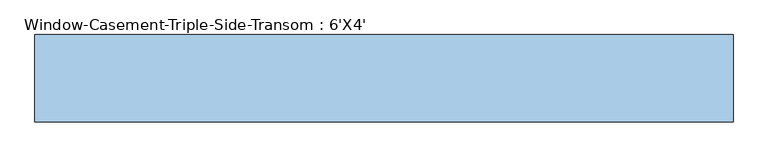
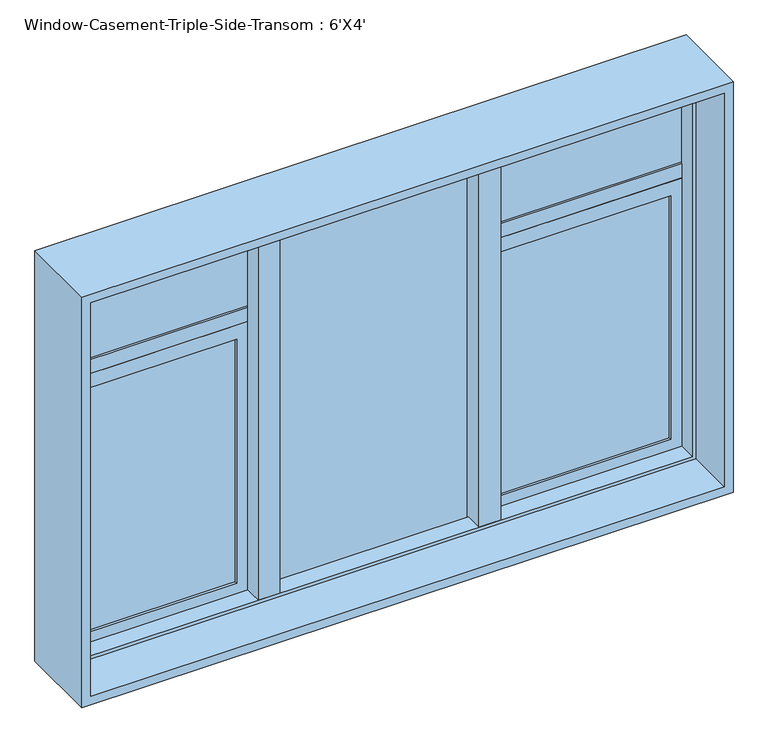
"""IFC4 building model written with IfcOpenShell, lengths in millimetres: window geometry, Window-Casement-Triple-Side-Transom : 6'X4'."""

from ifc_helpers import new_model, si_unit, frame, origin, place, context, project, spatial, polyline, outline, extrude, faceted_brep, source, transform, mapped, element, save


def window_casement_triple_side_transom_6_x4_596ba82f(model_context):
    return source(origin(), model_context, "Body", "SolidModel", [
        faceted_brep([(-889.0, 73.025, 2108.2), (-889.0, 114.3, 2108.2), (889.0, 114.3, 2108.2), (889.0, 73.025, 2108.2), (-878.8796875, 22.225, 2098.0796875), (-878.8796875, 73.025, 2098.0796875), (878.8796875, 73.025, 2098.0796875), (878.8796875, 22.225, 2098.0796875), (-889.0, -114.3, 2108.2), (-889.0, 22.225, 2108.2), (889.0, 22.225, 2108.2), (889.0, -114.3, 2108.2), (-914.4, 114.3, 2133.6), (-914.4, -114.3, 2133.6), (914.4, -114.3, 2133.6), (914.4, 114.3, 2133.6), (889.0, 114.3, 939.8), (889.0, 73.025, 939.8), (878.8796875, 73.025, 949.9203125), (878.8796875, 22.225, 949.9203125), (889.0, 22.225, 939.8), (889.0, -114.3, 939.8), (914.4, -114.3, 914.4), (914.4, 114.3, 914.4), (-889.0, 114.3, 939.8), (-889.0, 73.025, 939.8), (-878.8796875, 73.025, 949.9203125), (-878.8796875, 22.225, 949.9203125), (-889.0, 22.225, 939.8), (-889.0, -114.3, 939.8), (-914.4, -114.3, 914.4), (-914.4, 114.3, 914.4)], [[[0, 1, 2, 3]], [[4, 5, 6, 7]], [[8, 9, 10, 11]], [[12, 13, 14, 15]], [[3, 2, 16, 17]], [[7, 6, 18, 19]], [[11, 10, 20, 21]], [[15, 14, 22, 23]], [[17, 16, 24, 25]], [[19, 18, 26, 27]], [[21, 20, 28, 29]], [[23, 22, 30, 31]], [[25, 24, 1, 0]], [[3, 17, 25, 0], [5, 26, 18, 6]], [[27, 26, 5, 4]], [[9, 28, 20, 10], [7, 19, 27, 4]], [[29, 28, 9, 8]], [[13, 30, 22, 14], [11, 21, 29, 8]], [[31, 30, 13, 12]], [[15, 23, 31, 12], [1, 24, 16, 2]]]),
        extrude(outline(polyline([(-279.4, 111.125), (-279.4, 22.225), (-340.3203125, 22.225), (-340.3203125, 73.025), (-330.2, 73.025), (-330.2, 111.125), (-279.4, 111.125)])), frame((0.0, 0.0, 939.8), z_axis=(0.0, 0.0, 1.0), x_axis=(1.0, 0.0, 0.0)), (0.0, 0.0, 1.0), 1168.4),
        extrude(outline(polyline([(330.2, 111.125), (330.2, 73.025), (340.3203125, 73.025), (340.3203125, 22.225), (279.4, 22.225), (279.4, 111.125), (330.2, 111.125)])), frame((0.0, 0.0, 939.8), z_axis=(0.0, 0.0, 1.0), x_axis=(1.0, 0.0, 0.0)), (0.0, 0.0, 1.0), 1168.4),
        extrude(outline(polyline([(1746.9048438, 330.2), (939.8, 330.2), (939.8, 889.0), (1746.9048438, 889.0), (1746.9048438, 330.2)]), holes=[polyline([(1705.0345313, 847.1296875), (981.6703125, 847.1296875), (981.6703125, 372.0703125), (1705.0345313, 372.0703125), (1705.0345313, 847.1296875)])]), frame((0.0, 73.025, 0.0), z_axis=(0.0, 1.0, 0.0), x_axis=(0.0, 0.0, 1.0)), (0.0, 0.0, 1.0), 31.75),
        extrude(outline(polyline([(1746.9048438, -889.0), (939.8, -889.0), (939.8, -330.2), (1746.9048438, -330.2), (1746.9048438, -889.0)]), holes=[polyline([(1705.0345313, -372.0703125), (981.6703125, -372.0703125), (981.6703125, -847.1296875), (1705.0345313, -847.1296875), (1705.0345313, -372.0703125)])]), frame((0.0, 73.025, 0.0), z_axis=(0.0, 1.0, 0.0), x_axis=(0.0, 0.0, 1.0)), (0.0, 0.0, 1.0), 31.75),
        extrude(outline(polyline([(-372.0703125, 98.425), (-372.0703125, 92.075), (-847.1296875, 92.075), (-847.1296875, 98.425), (-372.0703125, 98.425)])), frame((0.0, 0.0, 981.6703125), z_axis=(0.0, 0.0, 1.0), x_axis=(1.0, 0.0, 0.0)), (0.0, 0.0, 1.0), 723.3642188),
        extrude(outline(polyline([(-372.0703125, 85.725), (-372.0703125, 79.375), (-847.1296875, 79.375), (-847.1296875, 85.725), (-372.0703125, 85.725)])), frame((0.0, 0.0, 981.6703125), z_axis=(0.0, 0.0, 1.0), x_axis=(1.0, 0.0, 0.0)), (0.0, 0.0, 1.0), 723.3642188),
        extrude(outline(polyline([(847.1296875, 98.425), (847.1296875, 92.075), (372.0703125, 92.075), (372.0703125, 98.425), (847.1296875, 98.425)])), frame((0.0, 0.0, 981.6703125), z_axis=(0.0, 0.0, 1.0), x_axis=(1.0, 0.0, 0.0)), (0.0, 0.0, 1.0), 723.3642188),
        extrude(outline(polyline([(847.1296875, 85.725), (847.1296875, 79.375), (372.0703125, 79.375), (372.0703125, 85.725), (847.1296875, 85.725)])), frame((0.0, 0.0, 981.6703125), z_axis=(0.0, 0.0, 1.0), x_axis=(1.0, 0.0, 0.0)), (0.0, 0.0, 1.0), 723.3642188),
        extrude(outline(polyline([(889.0, 104.775), (889.0, 73.025), (330.2, 73.025), (330.2, 104.775), (889.0, 104.775)])), frame((0.0, 0.0, 1746.9048438), z_axis=(0.0, 0.0, 1.0), x_axis=(1.0, 0.0, 0.0)), (0.0, 0.0, 1.0), 41.8703125),
        extrude(outline(polyline([(279.4, 98.425), (279.4, 92.075), (-279.4, 92.075), (-279.4, 98.425), (279.4, 98.425)])), frame((0.0, 0.0, 939.8), z_axis=(0.0, 0.0, 1.0), x_axis=(1.0, 0.0, 0.0)), (0.0, 0.0, 1.0), 1168.4),
        extrude(outline(polyline([(279.4, 85.725), (279.4, 79.375), (-279.4, 79.375), (-279.4, 85.725), (279.4, 85.725)])), frame((0.0, 0.0, 939.8), z_axis=(0.0, 0.0, 1.0), x_axis=(1.0, 0.0, 0.0)), (0.0, 0.0, 1.0), 1168.4),
        extrude(outline(polyline([(-330.2, 104.775), (-330.2, 73.025), (-889.0, 73.025), (-889.0, 104.775), (-330.2, 104.775)])), frame((0.0, 0.0, 1746.9048438), z_axis=(0.0, 0.0, 1.0), x_axis=(1.0, 0.0, 0.0)), (0.0, 0.0, 1.0), 41.8703125),
        extrude(outline(polyline([(-330.2, 98.425), (-330.2, 92.075), (-889.0, 92.075), (-889.0, 98.425), (-330.2, 98.425)])), frame((0.0, 0.0, 1788.7751562), z_axis=(0.0, 0.0, 1.0), x_axis=(1.0, 0.0, 0.0)), (0.0, 0.0, 1.0), 319.4248438),
        extrude(outline(polyline([(-330.2, 85.725), (-330.2, 79.375), (-889.0, 79.375), (-889.0, 85.725), (-330.2, 85.725)])), frame((0.0, 0.0, 1788.7751562), z_axis=(0.0, 0.0, 1.0), x_axis=(1.0, 0.0, 0.0)), (0.0, 0.0, 1.0), 319.4248438),
        extrude(outline(polyline([(889.0, 98.425), (889.0, 92.075), (330.2, 92.075), (330.2, 98.425), (889.0, 98.425)])), frame((0.0, 0.0, 1788.7751562), z_axis=(0.0, 0.0, 1.0), x_axis=(1.0, 0.0, 0.0)), (0.0, 0.0, 1.0), 319.4248438),
        extrude(outline(polyline([(889.0, 85.725), (889.0, 79.375), (330.2, 79.375), (330.2, 85.725), (889.0, 85.725)])), frame((0.0, 0.0, 1788.7751562), z_axis=(0.0, 0.0, 1.0), x_axis=(1.0, 0.0, 0.0)), (0.0, 0.0, 1.0), 319.4248438),
    ])


if __name__ == "__main__":
    model = new_model("IFC4")
    model_context = context("Model", 3, world=origin())
    ifc_project = project(units=[si_unit("LENGTHUNIT", "METRE", prefix="MILLI")], contexts=[model_context])
    site = spatial("IfcSite", under=ifc_project)
    building = spatial("IfcBuilding", under=site)
    placement = place(None, origin())
    window_casement_triple_side_transom_6_x4_shape = window_casement_triple_side_transom_6_x4_596ba82f(model_context)
    element("IfcWindow", 1, ObjectType="Window-Casement-Triple-Side-Transom : 6'X4'", at=placement, inside=building, context=model_context, shape_type="MappedRepresentation", body=[
        mapped(window_casement_triple_side_transom_6_x4_shape, transform((0.0, 0.0, 0.0), x_axis=(1.0, 0.0, 0.0), y_axis=(0.0, 1.0, 0.0), z_axis=(0.0, 0.0, 1.0))),
    ])
    save(model, "model.ifc")

# Revit data of these elements
# Type "Window-Casement-Triple-Side-Transom : 6'X4'"
#   Type Mark = "23"
#   Fire Rating = "0.5h"
#   Assembly Code = "B2020100"
#   Analytic Construction = "Double glazing - domestic"
#   Window Width = 2' - 0"
#   Window Inset [instance default] = 0' - 0 5/8"
#   Wall Thickness [instance default] = 0' - 6"
#   Visual Light Transmittance = 0.81
#   Transom Height Ratio = 0.3
#   Thermal Resistance (R) = 1.8146 (h·ft²·°F)/BTU
#   Solar Heat Gain Coefficient = 0.76
#   Rough Width = 6' - 0 1/2"
#   Rough Height = 4' - 0 1/2"
#   Open Window Height = 2' - 9.6"
#   Heat Transfer Coefficient (U) = 0.5511 BTU/(h·ft²·°F)
#   Height = 4' - 0"
#   Transom Height = 1' - 2.4"
#   Frame Gap 3 [instance default] = 0' - 1 83/128"
#   Frame Gap 2 [instance default] = 0' - 0 5/8"
#   Frame Gap 1 = 0' - 1 51/128"
#   Default Sill Height = 3' - 0"
#   Width = 6' - 0"
#   Frame Material = Metal - Aluminum
#   Glass Panel Material = Glass
#   Wall Closure = (empty or 0)
# Element 1 (IfcWindow, "Window-Casement-Triple-Side-Transom : 6'X4'")
#   Wall Thickness = 0' - 9"
#   Materials on its faces: "Metal - Aluminum", "Glass"
# Materials
#   "Metal - Aluminum": class "Metal", colour RGB 247 247 247, transparency 0
#   "Glass": class "Glass", colour RGB 0 128 192, transparency 0.75, Description = "Soda Lime Glass", Cost = 0
